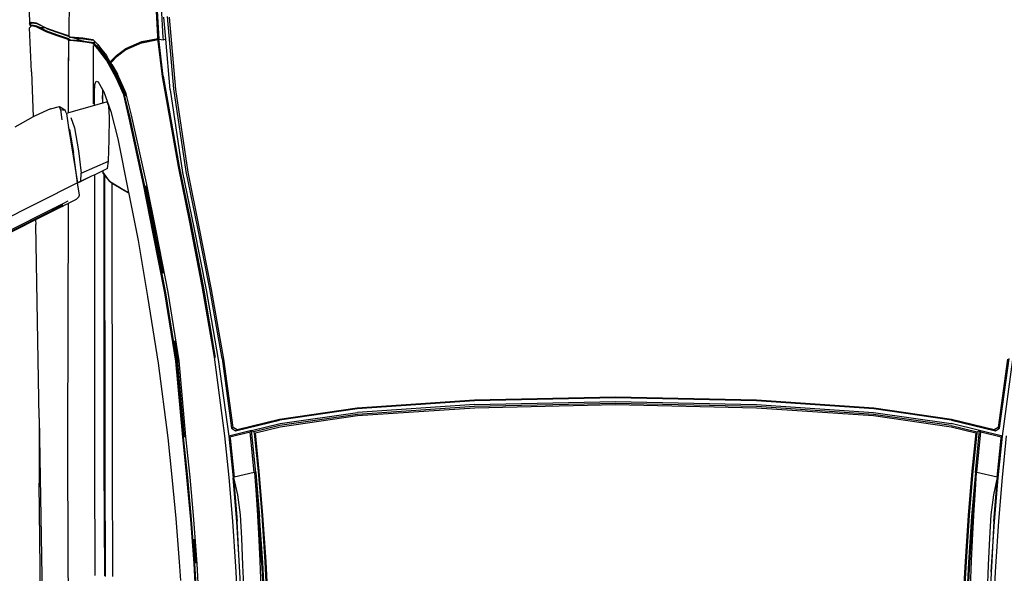
# Model space of a CAD drawing. Units: inches. Extents: x 22042254 to 25404563, y 17568978 to 17626777.
# Tile 29 of 45: x 22179810 to 22179875, y 17626295 to 17626332. Entities that reach past the tile are written whole.
import ezdxf

# ---------------------------------------------------------------- set-up
doc = ezdxf.new("R2010")
doc.units = ezdxf.units.IN
doc.header["$MEASUREMENT"] = 0
doc.layers.add('A-SITE-VEHI', color=8, linetype='Continuous', lineweight=18)
doc.layers.add('Edges', color=250, linetype='Continuous')

# ---------------------------------------------------------------- blocks, each defined once
blk = doc.blocks.new('Nissan Qashqai pl')
at = {"layer": 'Edges'}
for p, q in [((9.2669, 12.5088), (9.1605, 12.5233)), ((9.1612, 12.5208), (9.2656, 12.5065)), ((9.2789, 12.5131), (9.1617, 12.5292)), ((9.2783, 12.5191), (9.3422, 12.5126)), ((9.2656, 12.5065), (9.2669, 12.5088)), ((9.2656, 12.5065), (9.2694, 12.5006)), ((9.2707, 12.5028), (9.2669, 12.5088)), ((9.2789, 12.5131), (9.2704, 12.4783)), ((9.2724, 12.4804), (9.2799, 12.5114)), ((9.2799, 12.5114), (9.2789, 12.5131)), ((9.3427, 12.5066), (9.2789, 12.5131)), ((9.2819, 12.5112), (9.2799, 12.5114)), ((9.2803, 12.5116), (9.2822, 12.5118)), ((9.3418, 12.5051), (9.2819, 12.5112)), ((9.3418, 12.5051), (9.3346, 12.4741)), ((9.342, 12.5059), (9.3418, 12.5051)), ((9.3687, 12.5), (9.342, 12.5059)), ((9.4087, 12.5003), (9.342, 12.5059)), ((9.3422, 12.5126), (9.4088, 12.507)), ((9.4093, 12.5011), (9.3427, 12.5066)), ((9.4088, 12.507), (9.4782, 12.5024)), ((9.2694, 12.5006), (9.2535, 12.4354)), ((9.2543, 12.4356), (9.2707, 12.5028)), ((9.2707, 12.5028), (9.2694, 12.5006)), ((9.3992, 12.496), (9.3687, 12.5)), ((9.4347, 12.494), (9.3992, 12.496)), ((9.4087, 12.5003), (9.4688, 12.4968)), ((9.4785, 12.4965), (9.4093, 12.5011)), ((9.4761, 12.4919), (9.4347, 12.494)), ((9.4688, 12.4968), (9.4789, 12.4964)), ((9.5168, 12.4903), (9.4761, 12.4919)), ((9.4782, 12.5024), (9.5503, 12.4987)), ((9.4789, 12.4964), (9.4785, 12.4965)), ((9.4862, 12.4961), (9.4785, 12.4965)), ((9.4789, 12.4964), (9.4862, 12.4961)), ((9.4862, 12.4961), (9.514, 12.4949)), ((9.2704, 12.4783), (9.2598, 12.4348)), ((9.2629, 12.435), (9.2726, 12.4746)), ((9.2724, 12.4804), (9.2704, 12.4783)), ((9.2726, 12.4746), (9.2704, 12.4783)), ((9.3346, 12.4718), (9.2704, 12.4783)), ((9.3346, 12.4741), (9.2724, 12.4804)), ((9.2746, 12.4744), (9.2726, 12.4746)), ((9.333, 12.4685), (9.2746, 12.4744)), ((9.3346, 12.4741), (9.3344, 12.4733)), ((9.3344, 12.4733), (9.4017, 12.4677)), ((9.3344, 12.4733), (9.3611, 12.4715)), ((9.2649, 12.4348), (9.2741, 12.4725)), ((9.2741, 12.4725), (9.3326, 12.4666)), ((9.3326, 12.4666), (9.4, 12.4609)), ((9.4004, 12.4629), (9.333, 12.4685)), ((9.3346, 12.4718), (9.4018, 12.4661)), ((9.3611, 12.4715), (9.3918, 12.4695)), ((9.3918, 12.4695), (9.4276, 12.4674)), ((9.4, 12.4609), (9.4706, 12.4561)), ((9.4709, 12.4581), (9.4004, 12.4629)), ((9.4017, 12.4677), (9.472, 12.463)), ((9.4018, 12.4661), (9.472, 12.4614)), ((9.4276, 12.4674), (9.4694, 12.4654)), ((9.4694, 12.4654), (9.5105, 12.4637)), ((9.5446, 12.4542), (9.4709, 12.4581)), ((9.472, 12.463), (9.5454, 12.4591)), ((9.472, 12.4614), (9.5454, 12.4576)), ((9.4706, 12.4561), (9.5443, 12.4522)), ((9.2535, 12.4354), (9.2362, 12.3167)), ((9.2543, 12.4356), (9.2371, 12.3169)), ((9.2426, 12.3164), (9.2598, 12.4348)), ((9.2629, 12.435), (9.2457, 12.3164)), ((9.2476, 12.3163), (9.2649, 12.4348)), ((9.2362, 12.3167), (9.2241, 12.1376)), ((9.2371, 12.3169), (9.2249, 12.1376)), ((9.2305, 12.1375), (9.2426, 12.3164)), ((9.2457, 12.3164), (9.2335, 12.1374)), ((9.2355, 12.1374), (9.2476, 12.3163)), ((9.2241, 12.1376), (9.2195, 11.9221)), ((9.2249, 12.1376), (9.2203, 11.9221)), ((9.2259, 11.9221), (9.2305, 12.1375)), ((9.2335, 12.1374), (9.2289, 11.9221)), ((9.2308, 11.9221), (9.2355, 12.1374)), ((9.2195, 11.9221), (9.2241, 11.7066)), ((9.2203, 11.9221), (9.2249, 11.7065)), ((9.2305, 11.7067), (9.2259, 11.9221)), ((9.2289, 11.9221), (9.2335, 11.7067)), ((9.2355, 11.7068), (9.2308, 11.9221)), ((9.2241, 11.7066), (9.2362, 11.5274)), ((9.2249, 11.7065), (9.2371, 11.5273)), ((9.2305, 11.7067), (9.2426, 11.5277)), ((9.2335, 11.7067), (9.2457, 11.5277)), ((9.2476, 11.5278), (9.2355, 11.7068)), ((9.2362, 11.5274), (9.2535, 11.4087)), ((9.2371, 11.5273), (9.2543, 11.4085)), ((9.2598, 11.4093), (9.2426, 11.5277)), ((9.2457, 11.5277), (9.2629, 11.4092)), ((9.2649, 11.4094), (9.2476, 11.5278)), ((9.2535, 11.4087), (9.2694, 11.3436)), ((9.2707, 11.3414), (9.2543, 11.4085)), ((9.2704, 11.3659), (9.2598, 11.4093)), ((9.2629, 11.4092), (9.2726, 11.3695)), ((9.2741, 11.3716), (9.2649, 11.4094)), ((9.5443, 11.3919), (9.4706, 11.388)), ((9.4709, 11.3861), (9.5446, 11.39)), ((9.3326, 11.3776), (9.2741, 11.3716)), ((9.2746, 11.3697), (9.333, 11.3757)), ((9.4, 11.3832), (9.3326, 11.3776)), ((9.333, 11.3757), (9.4004, 11.3813)), ((9.4017, 11.3765), (9.3344, 11.3708)), ((9.3346, 11.3724), (9.4018, 11.378)), ((9.3918, 11.3747), (9.3611, 11.3727)), ((9.4276, 11.3767), (9.3918, 11.3747)), ((9.4706, 11.388), (9.4, 11.3832)), ((9.4004, 11.3813), (9.4709, 11.3861)), ((9.472, 11.3812), (9.4017, 11.3765)), ((9.472, 11.3828), (9.4018, 11.378)), ((9.4694, 11.3788), (9.4276, 11.3767)), ((9.5105, 11.3805), (9.4694, 11.3788)), ((9.5454, 11.3866), (9.472, 11.3828)), ((9.472, 11.3812), (9.5454, 11.3851)), ((9.3346, 11.3724), (9.2704, 11.3659)), ((9.2704, 11.3659), (9.2726, 11.3695)), ((9.2704, 11.3659), (9.2724, 11.3637)), ((9.2704, 11.3659), (9.2789, 11.331)), ((9.3346, 11.37), (9.2724, 11.3637)), ((9.2799, 11.3328), (9.2724, 11.3637)), ((9.2726, 11.3695), (9.2746, 11.3697)), ((9.3611, 11.3727), (9.3344, 11.3708)), ((9.3344, 11.3708), (9.3346, 11.37)), ((9.3346, 11.37), (9.3418, 11.3391)), ((9.3687, 11.3441), (9.3992, 11.3482)), ((9.3992, 11.3482), (9.4347, 11.3502)), ((9.4605, 11.3465), (9.4087, 11.3438)), ((9.4605, 11.3465), (9.4093, 11.3431)), ((9.4347, 11.3502), (9.4761, 11.3522)), ((9.514, 11.3492), (9.4605, 11.3465)), ((9.4761, 11.3522), (9.5168, 11.3539)), ((9.5503, 11.3455), (9.4782, 11.3418)), ((9.1605, 11.3208), (9.2669, 11.3354)), ((9.2656, 11.3376), (9.1612, 11.3233)), ((9.1617, 11.315), (9.2789, 11.331)), ((9.2694, 11.3436), (9.2656, 11.3376)), ((9.2669, 11.3354), (9.2656, 11.3376)), ((9.2669, 11.3354), (9.2707, 11.3414)), ((9.2694, 11.3436), (9.2707, 11.3414)), ((9.3422, 11.3316), (9.2783, 11.3251)), ((9.2789, 11.331), (9.3427, 11.3375)), ((9.2789, 11.331), (9.2799, 11.3327)), ((9.2799, 11.3328), (9.2819, 11.333)), ((9.2799, 11.3327), (9.2799, 11.3328)), ((9.2799, 11.3327), (9.2811, 11.3325)), ((9.2819, 11.333), (9.3418, 11.3391)), ((9.3418, 11.3391), (9.342, 11.3383)), ((9.342, 11.3383), (9.3687, 11.3441)), ((9.342, 11.3383), (9.4087, 11.3438)), ((9.4088, 11.3371), (9.3422, 11.3316)), ((9.4093, 11.3431), (9.3427, 11.3375)), ((9.4782, 11.3418), (9.4088, 11.3371)), ((9.1605, 11.3208), (9.0538, 11.3023)), ((9.1612, 11.3233), (9.0546, 11.3048)), ((9.0552, 11.2965), (9.1617, 11.315)), ((9.2783, 11.3251), (9.1584, 11.3091)), ((9.0538, 11.3023), (8.9583, 11.2833)), ((9.0546, 11.3048), (8.9591, 11.2859)), ((9.1584, 11.3091), (9.0495, 11.2906)), ((9.0497, 11.2918), (9.1586, 11.3104)), ((8.9591, 11.2859), (8.8754, 11.2687)), ((9.0495, 11.2906), (8.9521, 11.2715)), ((8.9522, 11.2728), (9.0497, 11.2918)), ((8.9598, 11.2775), (9.0552, 11.2965)), ((9.4739, 11.282), (9.5443, 11.2863)), ((8.8666, 11.2554), (8.9522, 11.2728)), ((8.9521, 11.2715), (8.8666, 11.2541)), ((8.9583, 11.2833), (8.8745, 11.266)), ((8.8761, 11.2602), (8.9598, 11.2775)), ((9.2801, 11.2648), (9.3418, 11.2713)), ((9.3418, 11.2713), (9.4064, 11.277)), ((9.4062, 11.2729), (9.3418, 11.2671)), ((9.4063, 11.2743), (9.3419, 11.2685)), ((9.4735, 11.2779), (9.4062, 11.2729)), ((9.4736, 11.2793), (9.4063, 11.2743)), ((9.4064, 11.277), (9.4739, 11.282)), ((9.4727, 11.2808), (9.4362, 11.278)), ((9.4727, 11.2808), (9.4732, 11.2808)), ((9.5437, 11.2822), (9.4735, 11.2779)), ((9.5438, 11.2836), (9.4736, 11.2793)), ((8.7287, 11.2307), (8.8666, 11.2554)), ((8.8666, 11.2541), (8.7292, 11.2295)), ((8.8745, 11.266), (8.7481, 11.2473)), ((8.8754, 11.2687), (8.7491, 11.2501)), ((8.7496, 11.2416), (8.8761, 11.2602)), ((9.0591, 11.2377), (9.1639, 11.2546)), ((9.1639, 11.2546), (9.2801, 11.2648)), ((9.2803, 11.2606), (9.1644, 11.2503)), ((9.2804, 11.262), (9.1645, 11.2518)), ((9.2804, 11.2635), (9.1668, 11.2533)), ((9.3418, 11.2671), (9.2803, 11.2606)), ((9.3419, 11.2685), (9.2804, 11.262)), ((9.4048, 11.2501), (9.471, 11.2554)), ((9.471, 11.2554), (9.4997, 11.2573)), ((8.7481, 11.2473), (8.6375, 11.2376)), ((8.7491, 11.2501), (8.6386, 11.2404)), ((8.7496, 11.2416), (8.6721, 11.2348)), ((9.1644, 11.2503), (9.06, 11.2335)), ((9.1645, 11.2518), (9.0601, 11.235)), ((9.133, 11.2481), (9.1647, 11.2532)), ((9.1647, 11.2532), (9.1668, 11.2533)), ((9.2814, 11.2377), (9.3416, 11.2442)), ((9.3416, 11.2442), (9.4048, 11.2501)), ((8.6203, 11.2213), (8.6721, 11.2241)), ((8.6699, 11.231), (8.622, 11.228)), ((8.6721, 11.2348), (8.6387, 11.2319)), ((8.6721, 11.2312), (8.6699, 11.231)), ((8.6721, 11.2241), (8.671, 11.2227)), ((8.6721, 11.2348), (8.6733, 11.2313)), ((8.6721, 11.2312), (8.6721, 11.2318)), ((8.6721, 11.2241), (8.6733, 11.2313)), ((8.6733, 11.2313), (8.6721, 11.2312)), ((8.7287, 11.2307), (8.6721, 11.2241)), ((8.6721, 11.2241), (8.6727, 11.2229)), ((8.6772, 11.1988), (8.6721, 11.2241)), ((8.7292, 11.2295), (8.6753, 11.2232)), ((9.0601, 11.235), (8.8941, 11.2023)), ((8.9679, 11.2201), (9.0591, 11.2377)), ((9.06, 11.2335), (8.9696, 11.2157)), ((8.9708, 11.2185), (9.03, 11.2304)), ((9.1676, 11.2229), (9.2814, 11.2377)), ((8.6683, 11.2226), (8.6197, 11.2201)), ((8.671, 11.2227), (8.6683, 11.2226)), ((8.6716, 11.2199), (8.671, 11.2227)), ((8.6759, 11.1982), (8.6716, 11.2199)), ((8.6753, 11.2232), (8.6727, 11.2229)), ((8.6777, 11.1984), (8.6727, 11.2229)), ((8.8918, 11.205), (8.9679, 11.2201)), ((8.9696, 11.2157), (8.8942, 11.2009)), ((8.8961, 11.204), (8.9318, 11.211)), ((8.9318, 11.211), (8.9704, 11.2185)), ((8.9704, 11.2185), (8.9708, 11.2185)), ((9.0656, 11.207), (9.1676, 11.2229)), ((8.6864, 11.1736), (8.6759, 11.1982)), ((8.6875, 11.1744), (8.6772, 11.1988)), ((8.6777, 11.1984), (8.6883, 11.1737)), ((8.7881, 11.1821), (8.8918, 11.205)), ((8.8941, 11.2023), (8.7925, 11.1802)), ((8.8942, 11.2009), (8.7931, 11.1789)), ((8.9797, 11.1924), (9.0656, 11.207)), ((8.7931, 11.1789), (8.7574, 11.1704)), ((8.7575, 11.1744), (8.7881, 11.1821)), ((8.7925, 11.1802), (8.7591, 11.1723)), ((8.9087, 11.1783), (8.9797, 11.1924)), ((8.697, 11.1592), (8.6864, 11.1736)), ((8.6979, 11.1603), (8.6875, 11.1744)), ((8.6883, 11.1737), (8.6987, 11.1597)), ((8.7508, 11.1722), (8.7257, 11.1609)), ((8.7529, 11.17), (8.7302, 11.1602)), ((8.7574, 11.1704), (8.7312, 11.1591)), ((8.7346, 11.1636), (8.7577, 11.1732)), ((8.7346, 11.1636), (8.7491, 11.1703)), ((8.7491, 11.1703), (8.7576, 11.1743)), ((8.7508, 11.1722), (8.7491, 11.1703)), ((8.7532, 11.1733), (8.7508, 11.1722)), ((8.7529, 11.17), (8.7577, 11.1732)), ((8.757, 11.1718), (8.7529, 11.17)), ((8.7532, 11.1733), (8.7575, 11.1744)), ((8.7587, 11.1722), (8.757, 11.1718)), ((8.7575, 11.1744), (8.7576, 11.1743)), ((8.7576, 11.1743), (8.7582, 11.1734)), ((8.7577, 11.1732), (8.7582, 11.1734)), ((8.7582, 11.1734), (8.759, 11.1725)), ((8.759, 11.1725), (8.7587, 11.1722)), ((8.7591, 11.1723), (8.7587, 11.1722)), ((8.759, 11.1725), (8.7591, 11.1723)), ((8.8245, 11.1613), (8.9063, 11.1779)), ((8.8893, 11.1486), (8.9021, 11.1697)), ((8.9041, 11.1717), (8.8927, 11.1528)), ((8.9021, 11.1697), (8.9063, 11.1779)), ((8.9075, 11.1781), (8.9041, 11.1717)), ((8.9063, 11.1779), (8.9075, 11.1781)), ((8.9075, 11.1781), (8.9087, 11.1783)), ((8.7055, 11.1514), (8.697, 11.1592)), ((8.6987, 11.1596), (8.6979, 11.1603)), ((8.7071, 11.15), (8.6981, 11.1446)), ((8.6987, 11.1597), (8.6988, 11.1596)), ((8.6987, 11.1596), (8.6988, 11.1596)), ((8.6996, 11.1588), (8.6987, 11.1596)), ((8.6988, 11.1596), (8.6996, 11.1588)), ((8.6996, 11.1588), (8.6996, 11.1588)), ((8.7062, 11.1527), (8.6996, 11.1588)), ((8.6996, 11.1588), (8.7062, 11.1527)), ((8.7302, 11.1602), (8.7032, 11.145)), ((8.7312, 11.1591), (8.7042, 11.144)), ((8.707, 11.15), (8.7055, 11.1514)), ((8.7067, 11.1522), (8.7062, 11.1527)), ((8.7083, 11.1508), (8.7067, 11.1522)), ((8.707, 11.15), (8.7083, 11.1508)), ((8.7071, 11.15), (8.707, 11.15)), ((8.707, 11.15), (8.707, 11.15)), ((8.7083, 11.1508), (8.7071, 11.15)), ((8.7075, 11.1487), (8.7346, 11.1636)), ((8.7083, 11.1507), (8.7102, 11.1519)), ((8.7083, 11.1508), (8.7083, 11.1507)), ((8.7102, 11.1519), (8.7108, 11.1523)), ((8.7108, 11.1523), (8.7257, 11.1609)), ((8.7108, 11.1523), (8.7248, 11.1605)), ((8.7248, 11.1605), (8.7257, 11.1609)), ((8.7524, 11.1401), (8.7828, 11.1508)), ((8.7916, 11.1488), (8.7748, 11.1475)), ((8.7828, 11.1508), (8.8245, 11.1613)), ((8.8259, 11.1483), (8.7916, 11.1488)), ((8.8913, 11.1506), (8.8893, 11.1486)), ((8.8927, 11.1528), (8.8913, 11.1506)), ((9.3225, 11.1531), (8.8927, 11.1528)), ((9.4936, 11.1538), (9.3225, 11.1531)), ((8.6805, 11.1309), (8.6884, 11.1371)), ((8.6818, 11.1288), (8.6902, 11.136)), ((8.6927, 11.1371), (8.6859, 11.132)), ((8.7042, 11.144), (8.687, 11.131)), ((8.6884, 11.1371), (8.6973, 11.144)), ((8.6884, 11.1371), (8.6917, 11.1371)), ((8.6902, 11.136), (8.6917, 11.1371)), ((8.6917, 11.1371), (8.7075, 11.1487)), ((8.6923, 11.1371), (8.6927, 11.1371)), ((8.7032, 11.145), (8.6927, 11.1371)), ((8.6973, 11.144), (8.698, 11.1446)), ((8.698, 11.1446), (8.6981, 11.1446)), ((8.7373, 11.1314), (8.7492, 11.1383)), ((8.7492, 11.1383), (8.7524, 11.1401)), ((8.7492, 11.1383), (8.7572, 11.1379)), ((8.7572, 11.1379), (8.7698, 11.1383)), ((8.7698, 11.1385), (8.7583, 11.1382)), ((8.7748, 11.1475), (8.7678, 11.1453)), ((8.7678, 11.1453), (8.7698, 11.1385)), ((8.7698, 11.1385), (8.7698, 11.1383)), ((8.7698, 11.1383), (8.7733, 11.126)), ((8.8585, 11.1473), (8.8259, 11.1483)), ((8.87, 11.1455), (8.8585, 11.1473)), ((8.8771, 11.1054), (8.8585, 11.1473)), ((8.87, 11.1455), (8.8734, 11.1385)), ((8.8734, 11.1385), (8.8793, 11.1261)), ((8.8734, 11.1385), (8.8768, 11.1385)), ((8.8893, 11.1486), (8.8751, 11.1387)), ((8.8751, 11.1387), (8.8768, 11.1385)), ((8.8768, 11.1385), (8.879, 11.1402)), ((8.879, 11.1402), (8.881, 11.1418)), ((8.879, 11.1402), (9.3198, 11.1403)), ((8.881, 11.1418), (8.8893, 11.1486)), ((9.3225, 11.1421), (8.881, 11.1418)), ((9.3198, 11.1403), (9.4922, 11.1409)), ((9.4936, 11.1428), (9.3225, 11.1421)), ((8.6703, 11.1081), (8.6727, 11.1235)), ((8.6714, 11.1088), (8.6737, 11.1245)), ((8.6727, 11.1235), (8.6737, 11.1245)), ((8.6737, 11.1245), (8.6746, 11.1253)), ((8.6805, 11.1309), (8.6746, 11.1253)), ((8.6746, 11.1253), (8.6785, 11.1253)), ((8.6777, 11.1246), (8.6755, 11.1099)), ((8.6788, 11.1237), (8.6764, 11.1083)), ((8.6785, 11.1253), (8.6777, 11.1246)), ((8.6815, 11.128), (8.6785, 11.1253)), ((8.687, 11.131), (8.6788, 11.1237)), ((8.6815, 11.128), (8.6818, 11.1288)), ((8.6817, 11.1282), (8.6815, 11.128)), ((8.6859, 11.132), (8.6817, 11.1282)), ((8.6817, 11.1282), (8.6818, 11.1288)), ((8.6818, 11.1238), (8.7026, 11.1238)), ((8.7026, 11.1238), (8.7026, 11.1239)), ((8.7026, 11.1238), (8.7072, 11.1239)), ((8.7072, 11.1239), (8.7072, 11.1239)), ((8.7072, 11.1239), (8.7273, 11.1239)), ((8.7273, 11.1239), (8.7273, 11.124)), ((8.7273, 11.1239), (8.7354, 11.124)), ((8.7354, 11.1241), (8.7354, 11.124)), ((8.7354, 11.124), (8.742, 11.124)), ((8.7361, 11.1283), (8.7373, 11.1314)), ((8.7415, 11.1265), (8.7361, 11.1283)), ((8.7534, 11.1257), (8.7415, 11.1265)), ((8.742, 11.1241), (8.742, 11.124)), ((8.742, 11.124), (8.742, 11.1241)), ((8.742, 11.124), (8.742, 11.124)), ((8.742, 11.124), (8.7426, 11.124)), ((8.7426, 11.1241), (8.7426, 11.124)), ((8.7426, 11.124), (8.7433, 11.124)), ((8.7433, 11.1241), (8.7433, 11.124)), ((8.7433, 11.124), (8.7711, 11.1241)), ((8.7711, 11.1241), (8.7516, 11.1241)), ((8.7718, 11.126), (8.7534, 11.1257)), ((8.7733, 11.126), (8.7718, 11.126)), ((8.7733, 11.126), (8.7849, 11.0859)), ((9.3194, 11.1262), (8.8793, 11.1261)), ((8.8793, 11.1261), (8.8815, 11.1214)), ((8.8815, 11.1214), (8.892, 11.0998)), ((8.8815, 11.1214), (8.8895, 11.1048)), ((9.4919, 11.1269), (9.3194, 11.1262)), ((8.6684, 11.0892), (8.6703, 11.1081)), ((8.6697, 11.0922), (8.6714, 11.1088)), ((8.6698, 11.0925), (8.6755, 11.1099)), ((8.6754, 11.1089), (8.6735, 11.0898)), ((8.6764, 11.1082), (8.6744, 11.0891)), ((8.6755, 11.1099), (8.6754, 11.1089)), ((8.6764, 11.1082), (8.6764, 11.1083)), ((8.8429, 11.1016), (8.8771, 11.1054)), ((8.8895, 11.1048), (8.8771, 11.1054)), ((8.8908, 11.1021), (8.8895, 11.1048)), ((8.8906, 11.1024), (8.8895, 11.1048)), ((8.6682, 11.087), (8.6684, 11.0888)), ((8.6684, 11.0888), (8.6684, 11.0892)), ((8.6684, 11.0888), (8.6685, 11.089)), ((8.6692, 11.0876), (8.6697, 11.0922)), ((8.6697, 11.0922), (8.6698, 11.0925)), ((8.6735, 11.0898), (8.6733, 11.0875)), ((8.6744, 11.0891), (8.6742, 11.0866)), ((8.7917, 11.0895), (8.8075, 11.0955)), ((8.807, 11.0862), (8.8918, 11.0997)), ((8.8075, 11.0955), (8.8429, 11.1016)), ((8.8102, 11.0874), (8.8455, 11.0936)), ((8.8918, 11.0997), (8.8455, 11.0936)), ((8.8906, 11.1024), (8.8911, 11.1013)), ((8.892, 11.0998), (8.8908, 11.1021)), ((8.8911, 11.1013), (8.8919, 11.0997)), ((8.8911, 11.1013), (8.8919, 11.0998)), ((8.8919, 11.0997), (8.8911, 11.1013)), ((8.8919, 11.0997), (8.8918, 11.0997)), ((8.8918, 11.0997), (9.0186, 10.8486)), ((8.892, 11.0998), (8.8919, 11.0998)), ((8.8919, 11.0998), (8.8919, 11.0997)), ((8.8919, 11.0997), (8.8919, 11.0997)), ((8.9106, 11.1029), (8.892, 11.0998)), ((8.892, 11.0998), (8.892, 11.0998)), ((8.9131, 11.102), (8.9106, 11.1029)), ((8.9171, 11.0978), (8.9131, 11.102)), ((8.9171, 11.0978), (8.917, 11.0974)), ((8.9171, 11.0978), (8.9233, 11.0855)), ((8.5326, 11.0874), (8.6675, 11.0866)), ((8.6606, 11.0674), (8.6667, 11.0857)), ((8.6616, 11.0683), (8.6675, 11.0862)), ((8.6718, 11.0868), (8.6657, 11.0684)), ((8.6667, 11.0857), (8.6675, 11.0862)), ((8.6728, 11.0858), (8.6667, 11.0675)), ((8.6674, 11.0864), (8.6675, 11.0865)), ((8.6675, 11.0865), (8.6675, 11.0866)), ((8.6676, 11.0866), (8.6675, 11.0866)), ((8.6675, 11.0862), (8.6679, 11.0864)), ((8.6676, 11.0864), (8.6677, 11.0866)), ((8.6677, 11.0866), (8.6676, 11.0866)), ((8.6682, 11.0866), (8.6677, 11.0866)), ((8.6679, 11.0864), (8.6682, 11.0866)), ((8.6692, 11.0876), (8.6682, 11.0866)), ((8.6682, 11.087), (8.6692, 11.0876)), ((8.6682, 11.0866), (8.6682, 11.087)), ((8.6729, 11.0874), (8.6718, 11.0868)), ((8.674, 11.0864), (8.6728, 11.0858)), ((8.6733, 11.0875), (8.6729, 11.0874)), ((8.6742, 11.0866), (8.674, 11.0864)), ((8.6744, 11.0866), (8.6742, 11.0866)), ((8.6742, 11.0858), (8.6743, 11.086)), ((8.6744, 11.0864), (8.6744, 11.0866)), ((8.6773, 11.0865), (8.6744, 11.0866)), ((8.6791, 11.0864), (8.677, 11.0864)), ((8.6791, 11.0865), (8.6773, 11.0865)), ((8.6791, 11.0865), (8.6791, 11.0864)), ((8.6878, 11.0864), (8.6791, 11.0865)), ((8.7205, 11.0863), (8.6791, 11.0864)), ((8.6878, 11.0864), (8.6791, 11.0864)), ((8.6878, 11.0865), (8.6878, 11.0864)), ((8.6911, 11.0864), (8.6878, 11.0864)), ((8.7205, 11.0863), (8.6911, 11.0864)), ((8.7849, 11.0859), (8.7205, 11.0863)), ((8.7751, 11.0723), (8.7779, 11.0773)), ((8.7798, 11.0739), (8.7751, 11.0723)), ((8.7779, 11.0773), (8.7807, 11.0812)), ((8.7798, 11.0739), (8.7807, 11.0812)), ((8.7798, 11.0739), (8.7954, 11.0758)), ((8.7849, 11.0827), (8.7807, 11.0812)), ((8.7849, 11.0859), (8.7856, 11.0834)), ((8.7849, 11.0827), (8.7858, 11.0828)), ((8.7858, 11.0828), (8.7856, 11.0834)), ((8.7858, 11.0828), (8.807, 11.0862)), ((8.8102, 11.0874), (8.807, 11.0862)), ((8.9232, 11.0779), (8.9194, 11.0854)), ((9.0333, 10.8597), (8.9232, 11.0779)), ((8.9233, 11.0855), (9.2886, 11.0848)), ((8.925, 11.0821), (8.9233, 11.0855)), ((8.928, 11.0762), (8.925, 11.0821)), ((9.0386, 10.8534), (8.9254, 11.0778)), ((8.928, 11.0762), (8.9483, 11.0359)), ((9.2886, 11.0848), (9.4673, 11.0852)), ((9.4673, 11.0852), (9.6358, 11.0866)), ((8.6546, 11.0516), (8.6606, 11.0674)), ((8.6556, 11.0524), (8.6616, 11.0683)), ((8.6657, 11.0684), (8.6598, 11.0529)), ((8.6667, 11.0675), (8.6608, 11.0521)), ((8.7785, 11.0587), (8.7751, 11.0723)), ((8.7785, 11.0587), (8.7891, 11.0353)), ((8.6472, 11.0366), (8.6546, 11.0516)), ((8.6482, 11.0375), (8.655, 11.0513)), ((8.6608, 11.0521), (8.6534, 11.0369)), ((8.6598, 11.0529), (8.655, 11.0432)), ((8.655, 11.0513), (8.6556, 11.0524)), ((8.655, 11.0513), (8.655, 11.0432)), ((9.2517, 11.0411), (9.5372, 11.0459)), ((9.641, 11.045), (9.351, 11.0411)), ((8.646, 11.0289), (8.6468, 11.0337)), ((8.6489, 11.0263), (8.646, 11.0289)), ((8.6468, 11.0337), (8.6472, 11.0366)), ((8.647, 11.03), (8.6468, 11.0337)), ((8.647, 11.03), (8.6482, 11.0375)), ((8.6498, 11.0273), (8.647, 11.03)), ((8.6527, 11.0286), (8.6489, 11.0263)), ((8.6524, 11.0289), (8.6498, 11.0273)), ((8.6524, 11.0378), (8.651, 11.0302)), ((8.651, 11.0302), (8.652, 11.0292)), ((8.6534, 11.0369), (8.652, 11.0292)), ((8.652, 11.0292), (8.6524, 11.0289)), ((8.655, 11.0432), (8.6524, 11.0378)), ((8.6524, 11.0289), (8.6527, 11.0286)), ((8.6527, 11.0286), (8.6537, 11.0275)), ((8.7222, 11.0298), (8.6547, 11.0265)), ((8.7222, 11.0298), (8.7908, 11.0322)), ((8.7891, 11.0353), (8.7908, 11.0322)), ((8.7908, 11.0322), (8.8066, 11.0041)), ((8.9483, 11.0359), (8.9552, 11.0361)), ((8.9483, 11.0359), (9.0343, 10.8656)), ((9.2517, 11.0411), (8.9552, 11.0361)), ((9.2517, 11.0411), (9.351, 11.0411)), ((8.5838, 11.0251), (8.6489, 11.0263)), ((8.6547, 11.0265), (8.6537, 11.0275)), ((8.6537, 11.0275), (8.6537, 11.0275))]:
    blk.add_line(p, q, dxfattribs=at)
blk = doc.blocks.new('CAR')
blk.add_blockref('Nissan Qashqai pl', (-9.7433, -11.9151))

msp = doc.modelspace()

# ---------------------------------------------------------------- block references
at = {"layer": 'A-SITE-VEHI', "xscale": 43.56002006885659, "yscale": 43.56002006885659, "zscale": 43.56002006885659, "rotation": 270}
msp.add_blockref('CAR', (22179848.861, 17626284.325), dxfattribs=at)

doc.saveas('drawing.dxf')
